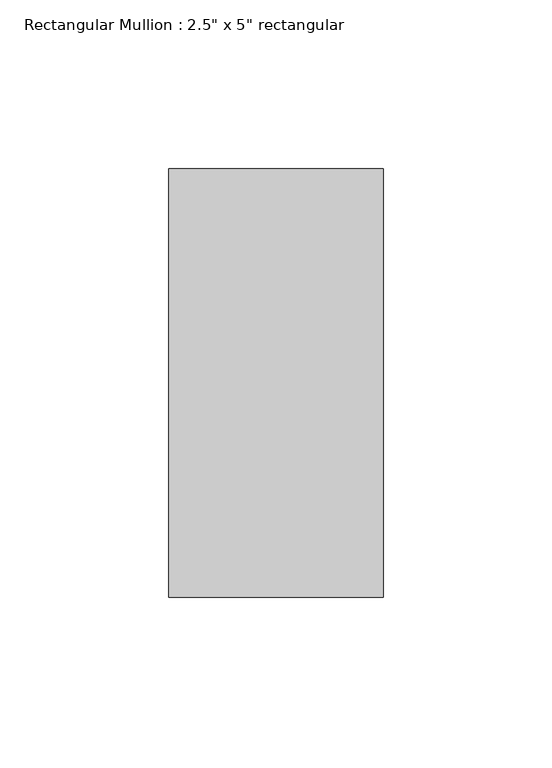
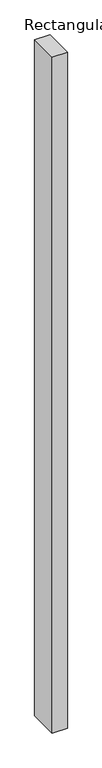
"""IFC4 building model written with IfcOpenShell, lengths in millimetres: member geometry."""

from ifc_helpers import new_model, si_unit, frame, origin, place, context, project, spatial, polyline, outline, extrude, source, transform, mapped, element, save


def member_56b0c076(model_context):
    return source(origin(), model_context, "Body", "SweptSolid", [
        extrude(outline(polyline([(0.0, 63.5), (0.0, -63.5), (-63.5, -63.5), (-63.5, 63.5), (0.0, 63.5)])), frame((0.0, 0.0, -2994.5946513), z_axis=(0.0, 0.0, 1.0), x_axis=(1.0, 0.0, 0.0)), (0.0, 0.0, 1.0), 2994.5946513),
    ])


if __name__ == "__main__":
    model = new_model("IFC4")
    model_context = context("Model", 3, world=origin())
    ifc_project = project(units=[si_unit("LENGTHUNIT", "METRE", prefix="MILLI")], contexts=[model_context])
    site = spatial("IfcSite", under=ifc_project)
    building = spatial("IfcBuilding", under=site)
    placement = place(None, origin())
    member_shape = member_56b0c076(model_context)
    element("IfcMember", 1, ObjectType="Rectangular Mullion : 2.5\" x 5\" rectangular", at=placement, inside=building, context=model_context, shape_type="MappedRepresentation", body=[
        mapped(member_shape, transform((0.0, 0.0, 0.0), x_axis=(1.0, 0.0, 0.0), y_axis=(0.0, 1.0, 0.0), z_axis=(0.0, 0.0, 1.0))),
    ])
    save(model, "model.ifc")

# Revit data of these elements
# Type "Rectangular Mullion : 2.5\" x 5\" rectangular"
#   built-in parameter 1007304 = 0.416667 (stored number, unit not read)
#   built-in parameter 1007301 = 0.104167 (stored number, unit not read)
#   built-in parameter 1007300 = 0.104167 (stored number, unit not read)
# Element 1 (IfcMember, "Rectangular Mullion : 2.5\" x 5\" rectangular")
#   Materials on its faces: "Aluminum"
# Materials
#   "Aluminum": class "Metal", colour RGB 247 247 247, transparency 0, Description = "Aluminum 6061", Cost = 0
